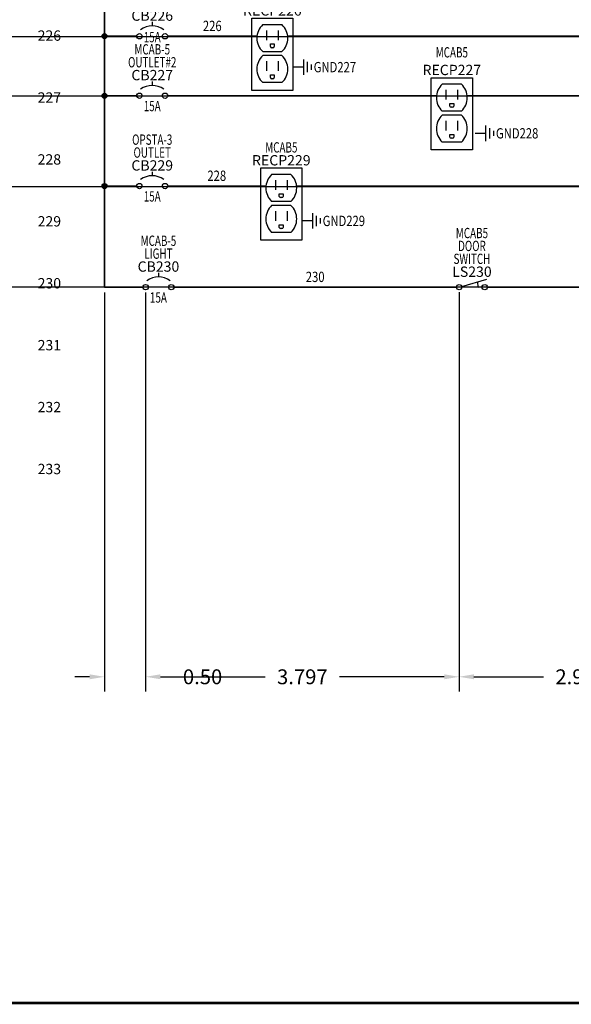
# Model space of a CAD drawing. Extents: x 0 to 33.5, y 0 to 22.4.
# Tile 6 of 8: x 19.9 to 26.6, y 0 to 11.9. Entities that reach past the tile are written whole.
import ezdxf
from ezdxf.enums import TextEntityAlignment as Align

# ---------------------------------------------------------------- set-up
doc = ezdxf.new("R2010")
doc.units = 0
doc.header["$MEASUREMENT"] = 0
for name, color, linetype, lineweight in [('A-ANNO-DIMS', 2, 'Continuous', 18), ('E-ANNO-TEXT', 3, 'Continuous', 18), ('MISC', 7, 'Continuous', 13), ('SYMS', 7, 'Continuous', 25), ('TITLE', 7, 'Continuous', 35), ('WIRENO', 72, 'Continuous', 18), ('WIRES', 7, 'Continuous', 35)]:
    doc.layers.add(name, color=color, linetype=linetype, lineweight=lineweight)
for name, color, linetype in [('DESC', 150, 'Continuous'), ('LOC', 8, 'Continuous'), ('TAGS', 150, 'Continuous')]:
    doc.layers.add(name, color=color, linetype=linetype)
doc.styles.add('ITALIC', font='ITALIC')
doc.styles.add('SIMPLEX', font='SIMPLEX')
doc.styles.add('WD', font='romans.shx')
doc.dimstyles.get("Standard").update_dxf_attribs({"dimtxt": 0.18, "dimasz": 0.18, "dimexe": 0.18, "dimexo": 0.0625, "dimgap": 0.09, "dimtad": 0, "dimtih": 1, "dimtoh": 1, "dimdec": 4, "dimzin": 0, "dimdsep": 46, "dimtxsty": 'Standard', "dimcen": 0.09, "dimadec": 0, "dimazin": 0, "dimtfac": 1, "dimtdec": 4, "dimtofl": 0, "dimtmove": 0, "dimatfit": 3, "dimfxl": 1, "dimtolj": 1, "dimtzin": 0, "dimarcsym": 0})

# ---------------------------------------------------------------- blocks, each defined once
blk = doc.blocks.new('NO_NUM_acade_title')
at = {"layer": 'TITLE', "const_width": 0.0312}
blk.add_lwpolyline([(30.594, 0.281), (30.594, 22.177), (30.344, 22.427), (0.281, 22.427), (0.031, 22.177), (0.031, 0.281), (0.281, 0.031), (30.344, 0.031)], close=True, dxfattribs=at)
at = {"layer": 'TITLE', "style": 'ITALIC'}
for tag, height, p in [('TITLE#1', 0.125, (32.156, 3.406)), ('TITLE#2', 0.125, (32.156, 3.204)), ('TITLE#3', 0.125, (32.156, 3.001)), ('TITLE#4', 0.125, (32.156, 2.799)), ('DWG#', 0.2, (32.156, 0.826))]:
    blk.add_attdef(tag, text='', height=height, dxfattribs=at).set_placement(p, align=Align.CENTER)
at = {"layer": 'TITLE', "style": 'SIMPLEX'}
blk.add_attdef('CAD#', (30.826, 1.958), '', height=0.0938, rotation=90, dxfattribs=at)
at = {"layer": 'TITLE'}
for tag, p, height, style in [('JOB#', (31.464, 1.644), 0.0938, 'SIMPLEX'), ('SCALE', (31.353, 1.344), 0.0938, 'SIMPLEX'), ('DATE', (32.408, 1.344), 0.0938, 'SIMPLEX'), ('SHTS', (32.532, 0.25), 0.2, 'ITALIC')]:
    blk.add_attdef(tag, p, '', height=height, dxfattribs=dict(at, style=style))
at = {"layer": 'TITLE', "style": 'ITALIC'}
blk.add_attdef('SH#', text='', height=0.2, dxfattribs=at).set_placement((31.881, 0.25), align=Align.RIGHT)
at = {"layer": 'TITLE', "flags": 9}
blk.add_attdef('WD_TB', (31.219, 0.031), '', height=0.125, dxfattribs=at)
blk = doc.blocks.new('WDDOT')
for radius in [0.03, 0.0187, 0.00929]:
    blk.add_circle((0, 0), radius)
blk = doc.blocks.new('HCB1')
blk.add_line((0, 0.173), (0, 0.126))
for centre in [(-0.155, 0), (0.155, 0)]:
    blk.add_circle(centre, 0.0322)
blk.add_arc((0, -0.109), 0.234, 53.1301, 126.8699)
at = {"style": 'WD', "width": 0.7}
for tag, p in [('INST', (0, 0.826)), ('LOC', (0, 0.656)), ('DESC1', (0, 0.5)), ('DESC2', (0, 0.344)), ('RATING1', (0, -0.188)), ('XREF', (0, -0.344))]:
    blk.add_attdef(tag, text='', height=0.125, dxfattribs=at).set_placement(p, align=Align.CENTER)
at = {"style": 'WD'}
blk.add_attdef('TAG1', text='', height=0.125, dxfattribs=at).set_placement((0, 0.188), align=Align.CENTER)
for tag, p in [('X2LINK', (0, 0.219)), ('X8LINK', (0, 0))]:
    blk.add_attdef(tag, p, '', height=0.01, dxfattribs=at)
for tag, p, height, flags in [('CONTACT', (0.205, 0.133), 0.01, 9), ('FAMILY', (0.205, 0.152), 0.01, 9), ('X4TERM01', (-0.188, 0), 0.0125, 1), ('X1TERM02', (0.188, 0), 0.0125, 1)]:
    blk.add_attdef(tag, p, '', height=height, dxfattribs=dict(at, flags=flags))
at = {"style": 'WD', "flags": 9}
for tag, p in [('ASSYCODE', (0.219, 0.062)), ('MFG', (0.228, 0.089)), ('CAT', (0.23, 0.108))]:
    blk.add_attdef(tag, text='', height=0.01, dxfattribs=at).set_placement(p, align=Align.CENTER)
at = {"style": 'WD', "flags": 8}
blk.add_attdef('TERM01', text='', height=0.125, dxfattribs=at).set_placement((-0.25, -0.031), align=Align.TOP_RIGHT)
blk.add_attdef('TERM02', text='', height=0.125, dxfattribs=at).set_placement((0.25, -0.031), align=Align.TOP_LEFT)
blk = doc.blocks.new('HCN1RDUP')
for p, q in [((-0.25, 0.219), (0.25, 0.219)), ((-0.25, -0.656), (-0.25, 0.219)), ((0.117, 0.14), (-0.117, 0.14)), ((0.25, 0.219), (0.25, -0.656)), ((-0.071, 0.071), (-0.071, -0.046)), ((0.07, 0.071), (0.07, -0.046)), ((-0.024, -0.093), (0.023, -0.093)), ((-0.024, -0.125), (-0.024, -0.093)), ((0.023, -0.093), (0.023, -0.125)), ((0.117, -0.187), (-0.117, -0.187)), ((0.117, -0.235), (-0.117, -0.235)), ((0.008, -0.14), (-0.009, -0.14)), ((-0.071, -0.304), (-0.071, -0.421)), ((0.07, -0.304), (0.07, -0.421)), ((-0.024, -0.468), (0.023, -0.468)), ((-0.024, -0.5), (-0.024, -0.468)), ((0.023, -0.468), (0.023, -0.5)), ((0.117, -0.562), (-0.117, -0.562)), ((0.008, -0.515), (-0.009, -0.515)), ((0.25, -0.656), (-0.25, -0.656))]:
    blk.add_line(p, q)
for centre, radius, start, end in [((0.039, -0.023), 0.226, 133.6028, 226.3972), ((-0.039, -0.023), 0.226, 313.6028, 46.3972), ((0.039, -0.398), 0.226, 133.6028, 226.3972), ((-0.009, -0.125), 0.015, 180, 270), ((0.008, -0.125), 0.015, 270, 0), ((-0.039, -0.398), 0.226, 313.6028, 46.3972), ((-0.009, -0.5), 0.015, 180, 270), ((0.008, -0.5), 0.015, 270, 0)]:
    blk.add_arc(centre, radius, start, end)
at = {"style": 'WD', "width": 0.7}
for tag, p in [('INST', (0, 0.875)), ('LOC', (0, 0.719)), ('DESC1', (0, 0.562)), ('DESC2', (0, 0.406))]:
    blk.add_attdef(tag, text='', height=0.125, dxfattribs=at).set_placement(p, align=Align.CENTER)
at = {"style": 'WD'}
blk.add_attdef('TAG1', text='', height=0.125, dxfattribs=at).set_placement((0, 0.25), align=Align.CENTER)
for tag, p, height, flags in [('FAMILY', (0.205, 0.152), 0.01, 9), ('X4TERM01', (-0.188, 0), 0.0125, 1), ('X1TERM02', (0.188, 0), 0.0125, 1), ('X8TERM03', (0, -0.14), 0.0125, 1), ('X4TERM04', (-0.188, -0.375), 0.0125, 1), ('X1TERM05', (0.188, -0.375), 0.0125, 1), ('X8TERM06', (0, -0.515), 0.0125, 1)]:
    blk.add_attdef(tag, p, '', height=height, dxfattribs=dict(at, flags=flags))
at = {"style": 'WD', "flags": 9}
for tag, p in [('ASSYCODE', (0.23, 0.071)), ('MFG', (0.228, 0.089)), ('CAT', (0.23, 0.108))]:
    blk.add_attdef(tag, text='', height=0.01, dxfattribs=at).set_placement(p, align=Align.CENTER)
at = {"style": 'WD', "flags": 8}
for tag, p in [('TERM01', (-0.281, -0.016)), ('TERM04', (-0.281, -0.391))]:
    blk.add_attdef(tag, text='', height=0.125, dxfattribs=at).set_placement(p, align=Align.TOP_RIGHT)
for tag, p in [('TERM02', (0.281, -0.016)), ('TERM05', (0.281, -0.391)), ('TERM06', (0.078, -0.688))]:
    blk.add_attdef(tag, text='', height=0.125, dxfattribs=at).set_placement(p, align=Align.TOP_LEFT)
at = {"style": 'WD', "width": 0.9}
blk.add_attdef('RATING1', text='', height=0.125, dxfattribs=at).set_placement((-0.281, -0.812), align=Align.RIGHT)
blk = doc.blocks.new('HGND2')
for p, q in [((0.125, 0), (0, 0)), ((0.125, 0.09375), (0.125, -0.09375)), ((0.171875, 0.0625), (0.171875, -0.0625)), ((0.21875, 0.03125), (0.21875, -0.03125))]:
    blk.add_line(p, q)
at = {"style": 'WD', "width": 0.8}
for tag, p in [('INST', (0.25, 0.3125)), ('LOC', (0.25, 0.15625)), ('TAG1', (0.25, 0)), ('DESC1', (0.25, -0.15625)), ('DESC2', (0.25, -0.3125))]:
    blk.add_attdef(tag, text='', height=0.125, dxfattribs=at).set_placement(p, align=Align.MIDDLE_LEFT)
at = {"style": 'WD', "flags": 1}
for tag in ['ASSYCODE', 'X4TERM01', 'CAT', 'MFG', 'FAMILY']:
    blk.add_attdef(tag, (0, 0), '', height=0.01, dxfattribs=at)
blk = doc.blocks.new('HLS12H')
for p, q in [((-0.124, 0.008), (0.179, 0.096)), ((-0.124, 0.008), (0.077, 0)), ((0.077, 0), (0.073, 0.065))]:
    blk.add_line(p, q)
for centre in [(-0.155, 0), (0.155, 0)]:
    blk.add_circle(centre, 0.0322)
at = {"style": 'WD', "width": 0.7}
for tag, p in [('INST', (0, 0.75)), ('LOC', (0, 0.594)), ('DESC1', (0, 0.437)), ('DESC2', (0, 0.281)), ('XREF', (0, -0.252)), ('WDTAGALT', (0, -0.406))]:
    blk.add_attdef(tag, text='', height=0.125, dxfattribs=at).set_placement(p, align=Align.CENTER)
at = {"style": 'WD'}
blk.add_attdef('TAG1', text='', height=0.125, dxfattribs=at).set_placement((0, 0.125), align=Align.CENTER)
for tag, p in [('X2LINK', (0, 0.125)), ('X8LINK', (0, -0.062))]:
    blk.add_attdef(tag, p, '', height=0.01, dxfattribs=at)
for tag, p, height, flags in [('X4TERM01', (-0.188, 0), 0.0125, 1), ('CONTACT', (0.038, 0.02), 0.01, 1), ('FAMILY', (0.038, 0.037), 0.01, 9), ('X1TERM02', (0.188, 0), 0.0125, 1)]:
    blk.add_attdef(tag, p, '', height=height, dxfattribs=dict(at, flags=flags))
at = {"style": 'WD', "flags": 9}
for tag, p in [('CAT', (0.063, -0.007)), ('ASSYCODE', (0.063, -0.046)), ('MFG', (0.063, -0.027))]:
    blk.add_attdef(tag, text='', height=0.01, dxfattribs=at).set_placement(p, align=Align.CENTER)
at = {"style": 'WD', "flags": 8}
blk.add_attdef('TERM01', text='', height=0.125, dxfattribs=at).set_placement((-0.25, -0.031), align=Align.TOP_RIGHT)
blk.add_attdef('TERM02', text='', height=0.125, dxfattribs=at).set_placement((0.25, -0.031), align=Align.TOP_LEFT)
blk = doc.blocks.new('WD_WNH')
at = {"style": 'WD', "width": 0.8}
blk.add_attdef('WIRENO', text='', height=0.125, dxfattribs=at).set_placement((0, 0.062), align=Align.CENTER)
at = {"style": 'WD', "flags": 1}
for tag, p in [('W01USER', (0, 0.078)), ('W02USER', (0, 0.07)), ('W03USER', (0, 0.062)), ('W04USER', (0, 0.055)), ('W05USER', (0, 0.047)), ('W06USER', (0, 0.039)), ('W07USER', (0, 0.031)), ('W08USER', (0, 0.023)), ('W09USER', (0, 0.016)), ('W10USER', (0, 0.008))]:
    blk.add_attdef(tag, text='', height=0.005, dxfattribs=at).set_placement(p, align=Align.CENTER)
blk = doc.blocks.new('*D52')
at = {"layer": 'A-ANNO-DIMS', "color": 0, "lineweight": -2, "transparency": 16777216}
for p, q in [((20.900842, 8.639801), (20.900842, 3.802917)), ((21.398489, 8.639801), (21.398489, 3.802917)), ((20.720842, 3.982917), (20.540842, 3.982917)), ((21.578489, 3.982917), (21.758489, 3.982917))]:
    blk.add_line(p, q, dxfattribs=at)
at = {"layer": 'A-ANNO-DIMS', "color": 0, "transparency": 16777216}
for points in [[(20.720842, 4.012917), (20.720842, 3.952917), (20.900842, 3.982917)], [(21.578489, 4.012917), (21.578489, 3.952917), (21.398489, 3.982917)]]:
    blk.add_solid(points, dxfattribs=at)
at = {"layer": 'Defpoints', "color": 0, "transparency": 16777216}
for p in [(20.900842, 8.702301), (21.398489, 8.702301), (21.398489, 3.982917)]:
    blk.add_point(p, dxfattribs=at)
at = {"layer": 'A-ANNO-DIMS', "color": 0, "transparency": 16777216, "insert": (22.088489, 3.982917), "char_height": 0.18, "attachment_point": 5}
blk.add_mtext('\\A1;0.50', dxfattribs=at)
blk = doc.blocks.new('*D53')
at = {"layer": 'A-ANNO-DIMS', "color": 0, "lineweight": -2, "transparency": 16777216}
for p, q in [((21.398489, 8.639801), (21.398489, 3.802917)), ((25.195375, 8.639671), (25.195375, 3.802917)), ((21.578489, 3.982917), (22.846932, 3.982917)), ((25.015375, 3.982917), (23.746932, 3.982917))]:
    blk.add_line(p, q, dxfattribs=at)
at = {"layer": 'A-ANNO-DIMS', "color": 0, "transparency": 16777216}
for points in [[(21.578489, 4.012917), (21.578489, 3.952917), (21.398489, 3.982917)], [(25.015375, 4.012917), (25.015375, 3.952917), (25.195375, 3.982917)]]:
    blk.add_solid(points, dxfattribs=at)
at = {"layer": 'Defpoints', "color": 0, "transparency": 16777216}
for p in [(21.398489, 8.702301), (25.195375, 8.702171), (25.195375, 3.982917)]:
    blk.add_point(p, dxfattribs=at)
at = {"layer": 'A-ANNO-DIMS', "color": 0, "transparency": 16777216, "insert": (23.296932, 3.982917), "char_height": 0.18, "attachment_point": 5}
blk.add_mtext('\\A1;3.797', dxfattribs=at)
blk = doc.blocks.new('*D54')
at = {"layer": 'A-ANNO-DIMS', "color": 0, "lineweight": -2, "transparency": 16777216}
for p, q in [((25.195, 8.64), (25.195, 3.803)), ((28.141, 8.64), (28.141, 3.803)), ((25.375, 3.983), (26.218, 3.983)), ((27.961, 3.983), (27.118, 3.983))]:
    blk.add_line(p, q, dxfattribs=at)
at = {"layer": 'A-ANNO-DIMS', "color": 0, "transparency": 16777216}
for points in [[(25.375, 4.013), (25.375, 3.953), (25.195, 3.983)], [(27.961, 4.013), (27.961, 3.953), (28.141, 3.983)]]:
    blk.add_solid(points, dxfattribs=at)
at = {"layer": 'Defpoints', "color": 0, "transparency": 16777216}
for p in [(25.195, 8.702), (28.141, 8.702), (28.141, 3.983)]:
    blk.add_point(p, dxfattribs=at)
at = {"layer": 'A-ANNO-DIMS', "color": 0, "transparency": 16777216, "insert": (26.668, 3.983), "char_height": 0.18, "attachment_point": 5}
blk.add_mtext('\\A1;2.946', dxfattribs=at)
blk = doc.blocks.new('*D57')
at = {"layer": 'A-ANNO-DIMS', "color": 0, "lineweight": -2, "transparency": 16777216}
for p, q in [((29.4322, 12.489774), (1.48, 12.489774)), ((1.66, 12.309774), (1.66, 11.913516)), ((29.435818, 11.733516), (1.48, 11.733516)), ((1.66, 11.733516), (1.66, 11.553516)), ((1.66, 11.553516), (1.48, 11.553516))]:
    blk.add_line(p, q, dxfattribs=at)
at = {"layer": 'A-ANNO-DIMS', "color": 0, "transparency": 16777216}
for points in [[(1.63, 12.309774), (1.69, 12.309774), (1.66, 12.489774)], [(1.63, 11.913516), (1.69, 11.913516), (1.66, 11.733516)]]:
    blk.add_solid(points, dxfattribs=at)
at = {"layer": 'Defpoints', "color": 0, "transparency": 16777216}
for p in [(29.4947, 12.489774), (1.66, 11.733516), (29.498318, 11.733516)]:
    blk.add_point(p, dxfattribs=at)
at = {"layer": 'A-ANNO-DIMS', "color": 0, "transparency": 16777216, "insert": (1.135, 11.553516), "char_height": 0.18, "attachment_point": 5}
blk.add_mtext('\\A1;0.76', dxfattribs=at)
blk = doc.blocks.new('*D58')
at = {"layer": 'A-ANNO-DIMS', "color": 0, "lineweight": -2, "transparency": 16777216}
for p, q in [((29.435818, 11.733516), (1.48, 11.733516)), ((1.66, 11.553516), (1.66, 11.194575)), ((29.438773, 11.014575), (1.48, 11.014575)), ((1.66, 11.014575), (1.66, 10.834575)), ((1.66, 10.834575), (1.48, 10.834575))]:
    blk.add_line(p, q, dxfattribs=at)
at = {"layer": 'A-ANNO-DIMS', "color": 0, "transparency": 16777216}
for points in [[(1.63, 11.553516), (1.69, 11.553516), (1.66, 11.733516)], [(1.63, 11.194575), (1.69, 11.194575), (1.66, 11.014575)]]:
    blk.add_solid(points, dxfattribs=at)
at = {"layer": 'Defpoints', "color": 0, "transparency": 16777216}
for p in [(29.498318, 11.733516), (1.66, 11.014575), (29.501273, 11.014575)]:
    blk.add_point(p, dxfattribs=at)
at = {"layer": 'A-ANNO-DIMS', "color": 0, "transparency": 16777216, "insert": (1.075, 10.834575), "char_height": 0.18, "attachment_point": 5}
blk.add_mtext('\\A1;0.719', dxfattribs=at)
blk = doc.blocks.new('*D59')
at = {"layer": 'A-ANNO-DIMS', "color": 0, "lineweight": -2, "transparency": 16777216}
for p, q in [((29.438773, 11.014575), (1.48, 11.014575)), ((1.66, 10.834575), (1.66, 10.646575)), ((1.66, 10.098575), (1.66, 10.286575)), ((29.435818, 9.918575), (1.48, 9.918575))]:
    blk.add_line(p, q, dxfattribs=at)
at = {"layer": 'A-ANNO-DIMS', "color": 0, "transparency": 16777216}
for points in [[(1.63, 10.834575), (1.69, 10.834575), (1.66, 11.014575)], [(1.63, 10.098575), (1.69, 10.098575), (1.66, 9.918575)]]:
    blk.add_solid(points, dxfattribs=at)
at = {"layer": 'Defpoints', "color": 0, "transparency": 16777216}
for p in [(29.501273, 11.014575), (1.66, 9.918575), (29.498318, 9.918575)]:
    blk.add_point(p, dxfattribs=at)
at = {"layer": 'A-ANNO-DIMS', "color": 0, "transparency": 16777216, "insert": (1.66, 10.466575), "char_height": 0.18, "attachment_point": 5}
blk.add_mtext('\\A1;1.096', dxfattribs=at)
blk = doc.blocks.new('*D60')
at = {"layer": 'A-ANNO-DIMS', "color": 0, "lineweight": -2, "transparency": 16777216}
for p, q in [((29.435818, 9.918575), (1.48, 9.918575)), ((1.66, 9.738575), (1.66, 9.490438)), ((1.66, 8.882301), (1.66, 9.130438)), ((29.4322, 8.702301), (1.48, 8.702301))]:
    blk.add_line(p, q, dxfattribs=at)
at = {"layer": 'A-ANNO-DIMS', "color": 0, "transparency": 16777216}
for points in [[(1.63, 9.738575), (1.69, 9.738575), (1.66, 9.918575)], [(1.63, 8.882301), (1.69, 8.882301), (1.66, 8.702301)]]:
    blk.add_solid(points, dxfattribs=at)
at = {"layer": 'Defpoints', "color": 0, "transparency": 16777216}
for p in [(29.498318, 9.918575), (1.66, 8.702301), (29.4947, 8.702301)]:
    blk.add_point(p, dxfattribs=at)
at = {"layer": 'A-ANNO-DIMS', "color": 0, "transparency": 16777216, "insert": (1.66, 9.310438), "char_height": 0.18, "attachment_point": 5}
blk.add_mtext('\\A1;1.22', dxfattribs=at)

msp = doc.modelspace()

# ---------------------------------------------------------------- linework, layer by layer
at = {"layer": 'WIRES'}
for p, q in [((20.9008, 13.2558), (20.9008, 8.7023)), ((20.9008, 11.7421), (21.2911, 11.7421)), ((21.6661, 11.7421), (22.7458, 11.7421)), ((23.1208, 11.7421), (29.4947, 11.7421)), ((20.9008, 11.0211), (21.2911, 11.0211)), ((21.6661, 11.0211), (24.9196, 11.0211)), ((25.2946, 11.0211), (29.4947, 11.0211)), ((20.9008, 9.9271), (21.2911, 9.9271)), ((21.6661, 9.9271), (22.8545, 9.9271)), ((23.2295, 9.9271), (29.4947, 9.9271)), ((21.3663, 8.7023), (20.9008, 8.7023)), ((25.1632, 8.7023), (21.7413, 8.7023)), ((28.1415, 8.7023), (25.5382, 8.7023))]:
    msp.add_line(p, q, dxfattribs=at)

# ---------------------------------------------------------------- block references
at = {"layer": 'SYMS'}
ref = msp.add_blockref('HCB1', (21.4786, 11.7421), dxfattribs=at)
ref.add_attrib('RATING1', '15A', dxfattribs={"layer": 'MISC', "height": 0.125, "style": 'WD', "width": 0.7}).set_placement((21.4786, 11.6685), align=Align.CENTER)
ref.add_attrib('DESC2', 'OUTLET#1', dxfattribs={"layer": 'DESC', "height": 0.125, "style": 'WD', "width": 0.7}).set_placement((21.4786, 12.0858), align=Align.CENTER)
ref.add_attrib('DESC1', 'MCAB-5', dxfattribs={"layer": 'DESC', "height": 0.125, "style": 'WD', "width": 0.7}).set_placement((21.4786, 12.2421), align=Align.CENTER)
ref.add_attrib('TAG1', 'CB226', dxfattribs={"layer": 'TAGS', "height": 0.125, "style": 'WD'}).set_placement((21.4786, 11.9296), align=Align.CENTER)
ref = msp.add_blockref('HCN1RDUP', (22.9333, 11.7421), dxfattribs=at)
ref.add_attrib('LOC', 'MCAB5', dxfattribs={"layer": 'LOC', "height": 0.125, "style": 'WD', "width": 0.7}).set_placement((22.9333, 12.2282), align=Align.CENTER)
ref.add_attrib('TAG1', 'RECP226', dxfattribs={"layer": 'TAGS', "height": 0.125, "style": 'WD'}).set_placement((22.9333, 11.9921), align=Align.CENTER)
for p in [(20.9008, 11.7421), (20.9008, 11.0211), (20.9008, 9.9271)]:
    msp.add_blockref('WDDOT', p, dxfattribs=at)
ref = msp.add_blockref('HCB1', (21.4786, 11.0211), dxfattribs=at)
ref.add_attrib('RATING1', '15A', dxfattribs={"layer": 'MISC', "height": 0.125, "style": 'WD', "width": 0.7}).set_placement((21.4786, 10.8336), align=Align.CENTER)
ref.add_attrib('DESC2', 'OUTLET#2', dxfattribs={"layer": 'DESC', "height": 0.125, "style": 'WD', "width": 0.7}).set_placement((21.4786, 11.3649), align=Align.CENTER)
ref.add_attrib('DESC1', 'MCAB-5', dxfattribs={"layer": 'DESC', "height": 0.125, "style": 'WD', "width": 0.7}).set_placement((21.4786, 11.5211), align=Align.CENTER)
ref.add_attrib('TAG1', 'CB227', dxfattribs={"layer": 'TAGS', "height": 0.125, "style": 'WD'}).set_placement((21.4786, 11.2086), align=Align.CENTER)
ref = msp.add_blockref('HCN1RDUP', (25.1071, 11.0211), dxfattribs=at)
ref.add_attrib('LOC', 'MCAB5', dxfattribs={"layer": 'LOC', "height": 0.125, "style": 'WD', "width": 0.7}).set_placement((25.1071, 11.4848), align=Align.CENTER)
ref.add_attrib('TAG1', 'RECP227', dxfattribs={"layer": 'TAGS', "height": 0.125, "style": 'WD'}).set_placement((25.1071, 11.2711), align=Align.CENTER)
ref = msp.add_blockref('HGND2', (23.1841, 11.3678), dxfattribs=at)
ref.add_attrib('TAG1', 'GND227', dxfattribs={"layer": 'TAGS', "height": 0.125, "style": 'WD', "width": 0.8}).set_placement((23.4341, 11.3678), align=Align.MIDDLE_LEFT)
ref = msp.add_blockref('HGND2', (25.3914, 10.5659), dxfattribs=at)
ref.add_attrib('TAG1', 'GND228', dxfattribs={"layer": 'TAGS', "height": 0.125, "style": 'WD', "width": 0.8}).set_placement((25.6414, 10.5659), align=Align.MIDDLE_LEFT)
ref = msp.add_blockref('HCB1', (21.4786, 9.9271), dxfattribs=at)
ref.add_attrib('RATING1', '15A', dxfattribs={"layer": 'MISC', "height": 0.125, "style": 'WD', "width": 0.7}).set_placement((21.4786, 9.7396), align=Align.CENTER)
ref.add_attrib('DESC2', 'OUTLET', dxfattribs={"layer": 'DESC', "height": 0.125, "style": 'WD', "width": 0.7}).set_placement((21.4786, 10.2709), align=Align.CENTER)
ref.add_attrib('DESC1', 'OPSTA-3', dxfattribs={"layer": 'DESC', "height": 0.125, "style": 'WD', "width": 0.7}).set_placement((21.4786, 10.4271), align=Align.CENTER)
ref.add_attrib('TAG1', 'CB229', dxfattribs={"layer": 'TAGS', "height": 0.125, "style": 'WD'}).set_placement((21.4786, 10.1146), align=Align.CENTER)
ref = msp.add_blockref('HCN1RDUP', (23.042, 9.9271), dxfattribs=at)
ref.add_attrib('LOC', 'MCAB5', dxfattribs={"layer": 'LOC', "height": 0.125, "style": 'WD', "width": 0.7}).set_placement((23.042, 10.3334), align=Align.CENTER)
ref.add_attrib('TAG1', 'RECP229', dxfattribs={"layer": 'TAGS', "height": 0.125, "style": 'WD'}).set_placement((23.042, 10.1771), align=Align.CENTER)
ref = msp.add_blockref('HGND2', (23.2928, 9.5051), dxfattribs=at)
ref.add_attrib('TAG1', 'GND229', dxfattribs={"layer": 'TAGS', "height": 0.125, "style": 'WD', "width": 0.8}).set_placement((23.5428, 9.5051), align=Align.MIDDLE_LEFT)
ref = msp.add_blockref('HLS12H', (25.3507, 8.7022), dxfattribs=at)
ref.add_attrib('LOC', 'MCAB5', dxfattribs={"layer": 'LOC', "height": 0.125, "style": 'WD', "width": 0.7}).set_placement((25.3507, 9.2959), align=Align.CENTER)
ref.add_attrib('DESC2', 'SWITCH', dxfattribs={"layer": 'DESC', "height": 0.125, "style": 'WD', "width": 0.7}).set_placement((25.3507, 8.9834), align=Align.CENTER)
ref.add_attrib('DESC1', 'DOOR', dxfattribs={"layer": 'DESC', "height": 0.125, "style": 'WD', "width": 0.7}).set_placement((25.3507, 9.1397), align=Align.CENTER)
ref.add_attrib('TAG1', 'LS230', dxfattribs={"layer": 'TAGS', "height": 0.125, "style": 'WD'}).set_placement((25.3507, 8.8272), align=Align.CENTER)
ref = msp.add_blockref('HCB1', (21.5538, 8.7023), dxfattribs=at)
ref.add_attrib('RATING1', '15A', dxfattribs={"layer": 'MISC', "height": 0.125, "style": 'WD', "width": 0.7}).set_placement((21.5538, 8.5148), align=Align.CENTER)
ref.add_attrib('DESC2', 'LIGHT', dxfattribs={"layer": 'DESC', "height": 0.125, "style": 'WD', "width": 0.7}).set_placement((21.5538, 9.0461), align=Align.CENTER)
ref.add_attrib('DESC1', 'MCAB-5', dxfattribs={"layer": 'DESC', "height": 0.125, "style": 'WD', "width": 0.7}).set_placement((21.5538, 9.2023), align=Align.CENTER)
ref.add_attrib('TAG1', 'CB230', dxfattribs={"layer": 'TAGS', "height": 0.125, "style": 'WD'}).set_placement((21.5538, 8.8898), align=Align.CENTER)
at = {"layer": 'TITLE'}
msp.add_blockref('NO_NUM_acade_title', (0, 0), dxfattribs=at)
at = {"layer": 'WIRENO'}
ref = msp.add_blockref('WD_WNH', (22.206, 11.7421), dxfattribs=at)
ref.add_attrib('WIRENO', '226', dxfattribs={"linetype": 'Continuous', "height": 0.125, "style": 'WD', "width": 0.8}).set_placement((22.206, 11.8046), align=Align.CENTER)
ref = msp.add_blockref('WD_WNH', (22.2603, 9.9271), dxfattribs=at)
ref.add_attrib('WIRENO', '228', dxfattribs={"linetype": 'Continuous', "height": 0.125, "style": 'WD', "width": 0.8}).set_placement((22.2603, 9.9896), align=Align.CENTER)
ref = msp.add_blockref('WD_WNH', (23.4522, 8.7023), dxfattribs=at)
ref.add_attrib('WIRENO', '230', dxfattribs={"linetype": 'Continuous', "height": 0.125, "style": 'WD', "width": 0.8}).set_placement((23.4522, 8.7648), align=Align.CENTER)

# ---------------------------------------------------------------- texts
at = {"layer": 'E-ANNO-TEXT', "style": 'WD'}
for s, p in [('226', (20.3748, 11.75)), ('227', (20.3748, 11)), ('228', (20.3748, 10.25)), ('229', (20.3748, 9.5)), ('230', (20.3748, 8.75)), ('231', (20.3748, 8)), ('232', (20.3748, 7.25)), ('233', (20.3748, 6.5))]:
    msp.add_text(s, height=0.125, dxfattribs=at).set_placement(p, align=Align.MIDDLE_RIGHT)

# ---------------------------------------------------------------- dimensions: what is measured, and where the dimension line sits
at = {"layer": 'A-ANNO-DIMS'}
for base, p1, p2, override, picture, middle in [((1.66, 11.7335), (29.4947, 12.4898), (29.4983, 11.7335), {"dimdec": 2, "dimlfac": 1, "dimrnd": 0, "dimzin": 0, "dimdsep": 46, "dimlunit": 2}, '*D57', (1.135, 11.5535)), ((1.66, 11.0146), (29.4983, 11.7335), (29.5013, 11.0146), {"dimdec": 3, "dimlfac": 1, "dimrnd": 0, "dimzin": 0, "dimdsep": 46, "dimlunit": 2}, '*D58', (1.075, 10.8346)), ((1.66, 9.9186), (29.5013, 11.0146), (29.4983, 9.9186), {"dimdec": 3, "dimlfac": 1, "dimrnd": 0, "dimzin": 0, "dimdsep": 46, "dimlunit": 2}, '*D59', (1.66, 10.4666)), ((1.66, 8.7023), (29.4983, 9.9186), (29.4947, 8.7023), {"dimdec": 2, "dimlfac": 1, "dimrnd": 0, "dimzin": 0, "dimdsep": 46, "dimlunit": 2}, '*D60', (1.66, 9.3104))]:
    dim = msp.add_linear_dim(base=base, p1=p1, p2=p2, angle=90, dimstyle='Standard', override=override, dxfattribs=at)
    dim.commit()
    dim.dimension.update_dxf_attribs({"geometry": picture, "text_midpoint": middle})
for base, p1, p2, override, picture, middle in [((21.3985, 3.9829), (20.9008, 8.7023), (21.3985, 8.7023), {"dimdec": 2, "dimlfac": 1, "dimrnd": 0, "dimzin": 0, "dimdsep": 46, "dimlunit": 2}, '*D52', (22.0885, 3.9829)), ((25.1954, 3.9829), (21.3985, 8.7023), (25.1954, 8.7022), {"dimdec": 3, "dimlfac": 1, "dimrnd": 0, "dimzin": 0, "dimdsep": 46, "dimlunit": 2}, '*D53', (23.2969, 3.9829)), ((28.1415, 3.9829), (25.1954, 8.7022), (28.1415, 8.7023), {"dimdec": 3, "dimlfac": 1, "dimrnd": 0, "dimzin": 0, "dimdsep": 46, "dimlunit": 2}, '*D54', (26.6684, 3.9829))]:
    dim = msp.add_linear_dim(base=base, p1=p1, p2=p2, dimstyle='Standard', override=override, dxfattribs=at)
    dim.commit()
    dim.dimension.update_dxf_attribs({"geometry": picture, "text_midpoint": middle})

doc.saveas('drawing.dxf')
